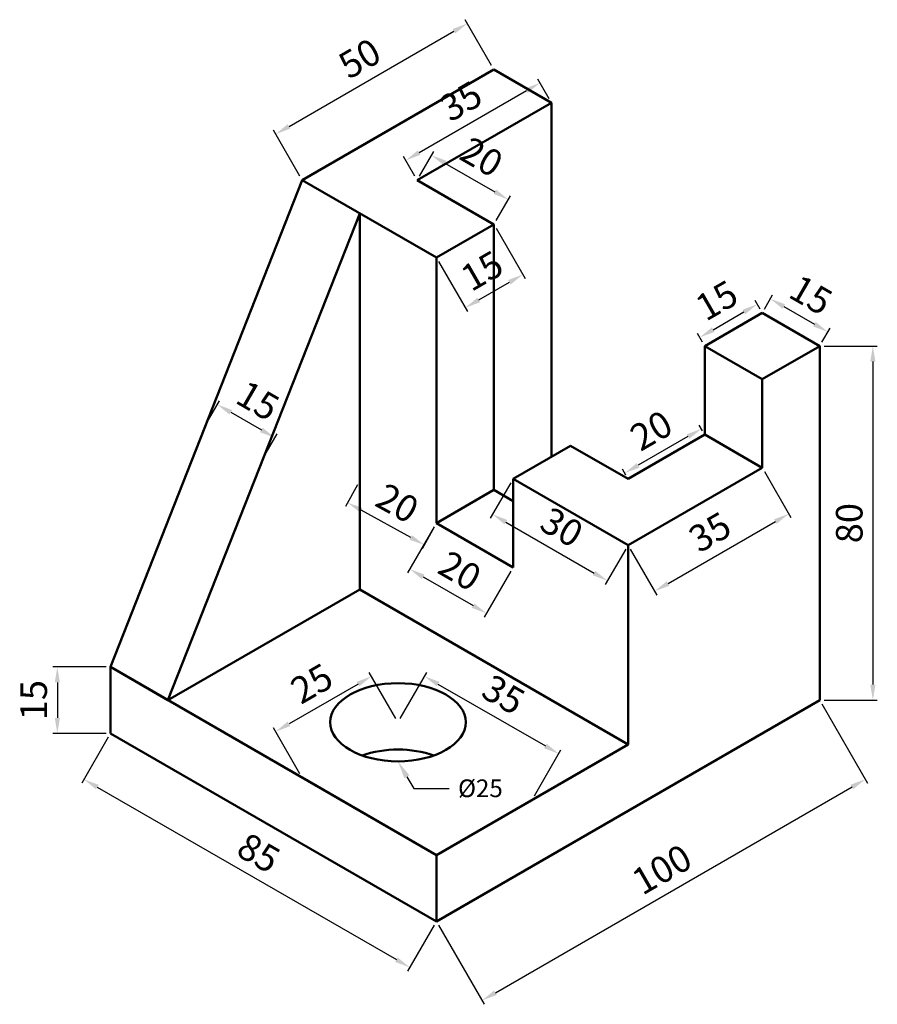
# Model space of a CAD drawing. Units: millimetres. Extents: x 2933 to 3127, y 771 to 994.
import ezdxf
from ezdxf import colors
from ezdxf.entities.mleader import LeaderData, LeaderLine
from ezdxf.math import Vec2, Vec3

# ---------------------------------------------------------------- set-up
doc = ezdxf.new("R2010")
doc.units = ezdxf.units.MM
for name, color, linetype, lineweight in [('M-DIMS', 3, 'Continuous', 25), ('M-OUTL', 7, 'Continuous', 50), ('M-TEXT', 7, 'Continuous', 25)]:
    doc.layers.add(name, color=color, linetype=linetype, lineweight=lineweight)
doc.styles.get("Standard").update_dxf_attribs({"font": 'arial.ttf'})
doc.dimstyles.new('AM_ISO$0', dxfattribs={"dimtxt": 6, "dimasz": 3.5, "dimexe": 1, "dimexo": 1, "dimgap": 1.5, "dimtad": 1, "dimdsep": 46, "dimtxsty": 'Standard', "dimcen": 0, "dimclrd": 256, "dimclre": 256, "dimclrt": 2, "dimadec": 0, "dimazin": 2, "dimtp": 0.1, "dimtm": 0.1, "dimtfac": 0.71, "dimtmove": 0, "dimatfit": 3, "dimfxl": 1, "dimlwd": -1, "dimlwe": -1, "dimarcsym": 1})

# ---------------------------------------------------------------- blocks, each defined once
blk = doc.blocks.new('*D3')
at = {"layer": 'Defpoints', "color": 0, "transparency": 16777216}
for p in [(3113.5, 839.77), (3123.82, 821.91), (3026.9, 789.77)]:
    blk.add_point(p, dxfattribs=at)
at = {"layer": 'M-DIMS', "color": 0, "linetype": 'ByBlock', "transparency": 16777216}
for p, q in [((3114, 838.9), (3124.32, 821.04)), ((3040.25, 773.66), (3120.79, 820.16)), ((3027.4, 788.9), (3037.71, 771.04))]:
    blk.add_line(p, q, dxfattribs=at)
at = {"layer": 'M-DIMS', "color": 0, "transparency": 16777216}
for points in [[(3120.49, 820.66), (3121.08, 819.65), (3123.82, 821.91)], [(3039.95, 774.16), (3040.54, 773.15), (3037.21, 771.91)]]:
    blk.add_solid(points, dxfattribs=at)
at = {"layer": 'M-DIMS', "color": 0, "transparency": 16777216, "insert": (3078.23, 800.86), "char_height": 6, "attachment_point": 5, "rotation": 30}
blk.add_mtext('100', dxfattribs=at)
blk = doc.blocks.new('*D4')
at = {"layer": 'Defpoints', "color": 0, "transparency": 16777216}
for p in [(3113.5, 919.77), (3113.5, 839.77), (3125.5, 839.77)]:
    blk.add_point(p, dxfattribs=at)
at = {"layer": 'M-DIMS', "color": 0, "linetype": 'ByBlock', "transparency": 16777216}
for p, q in [((3114.5, 919.77), (3126.5, 919.77)), ((3125.5, 916.27), (3125.5, 843.27)), ((3114.5, 839.77), (3126.5, 839.77))]:
    blk.add_line(p, q, dxfattribs=at)
at = {"layer": 'M-DIMS', "color": 0, "transparency": 16777216}
for points in [[(3124.92, 916.27), (3126.09, 916.27), (3125.5, 919.77)], [(3124.92, 843.27), (3126.09, 843.27), (3125.5, 839.77)]]:
    blk.add_solid(points, dxfattribs=at)
at = {"layer": 'M-DIMS', "color": 0, "transparency": 16777216, "insert": (3120.94, 879.77), "char_height": 6, "attachment_point": 5, "rotation": 90}
blk.add_mtext('80', dxfattribs=at)
blk = doc.blocks.new('*D5')
at = {"layer": 'Defpoints', "color": 0, "transparency": 16777216}
for p in [(2953.29, 832.27), (3026.9, 789.77), (3020.9, 779.38)]:
    blk.add_point(p, dxfattribs=at)
at = {"layer": 'M-DIMS', "color": 0, "linetype": 'ByBlock', "transparency": 16777216}
for p, q in [((2952.79, 831.4), (2946.79, 821.01)), ((2950.32, 820.13), (3017.87, 781.13)), ((3026.4, 788.9), (3020.4, 778.51))]:
    blk.add_line(p, q, dxfattribs=at)
at = {"layer": 'M-DIMS', "color": 0, "transparency": 16777216}
for points in [[(2950.61, 820.63), (2950.03, 819.62), (2947.29, 821.88)], [(3018.16, 781.63), (3017.58, 780.62), (3020.9, 779.38)]]:
    blk.add_solid(points, dxfattribs=at)
at = {"layer": 'M-DIMS', "color": 0, "transparency": 16777216, "insert": (2986.38, 804.58), "char_height": 6, "attachment_point": 5, "rotation": 330}
blk.add_mtext('85', dxfattribs=at)
blk = doc.blocks.new('*D6')
at = {"layer": 'Defpoints', "color": 0, "transparency": 16777216}
for p in [(2953.29, 847.27), (2941.29, 832.27), (2953.29, 832.27)]:
    blk.add_point(p, dxfattribs=at)
at = {"layer": 'M-DIMS', "color": 0, "linetype": 'ByBlock', "transparency": 16777216}
for p, q in [((2952.29, 847.27), (2940.29, 847.27)), ((2941.29, 843.77), (2941.29, 835.77)), ((2952.29, 832.27), (2940.29, 832.27))]:
    blk.add_line(p, q, dxfattribs=at)
at = {"layer": 'M-DIMS', "color": 0, "transparency": 16777216}
for points in [[(2940.71, 843.77), (2941.87, 843.77), (2941.29, 847.27)], [(2940.71, 835.77), (2941.87, 835.77), (2941.29, 832.27)]]:
    blk.add_solid(points, dxfattribs=at)
at = {"layer": 'M-DIMS', "color": 0, "transparency": 16777216, "insert": (2936.73, 839.77), "char_height": 6, "attachment_point": 5, "rotation": 90}
blk.add_mtext('15', dxfattribs=at)
blk = doc.blocks.new('*D7')
at = {"layer": 'Defpoints', "color": 0, "transparency": 16777216}
for p in [(3033.89, 992.66), (3039.89, 982.27), (2996.59, 957.27)]:
    blk.add_point(p, dxfattribs=at)
at = {"layer": 'M-DIMS', "color": 0, "linetype": 'ByBlock', "transparency": 16777216}
for p, q in [((3039.39, 983.14), (3033.39, 993.53)), ((2993.62, 969.41), (3030.86, 990.91)), ((2996.09, 958.14), (2990.09, 968.53))]:
    blk.add_line(p, q, dxfattribs=at)
at = {"layer": 'M-DIMS', "color": 0, "transparency": 16777216}
for points in [[(3030.57, 991.42), (3031.15, 990.41), (3033.89, 992.66)], [(2993.33, 969.92), (2993.91, 968.91), (2990.59, 967.66)]]:
    blk.add_solid(points, dxfattribs=at)
at = {"layer": 'M-DIMS', "color": 0, "transparency": 16777216, "insert": (3009.96, 984.11), "char_height": 6, "attachment_point": 5, "rotation": 30}
blk.add_mtext('50', dxfattribs=at)
blk = doc.blocks.new('*D8')
at = {"layer": 'Defpoints', "color": 0, "transparency": 16777216}
for p in [(3039.89, 947.27), (3026.9, 939.77), (3046.43, 935.94)]:
    blk.add_point(p, dxfattribs=at)
at = {"layer": 'M-DIMS', "color": 0, "linetype": 'ByBlock', "transparency": 16777216}
for p, q in [((3040.39, 946.4), (3046.93, 935.08)), ((3027.4, 938.9), (3033.94, 927.58)), ((3036.47, 930.19), (3043.4, 934.19))]:
    blk.add_line(p, q, dxfattribs=at)
at = {"layer": 'M-DIMS', "color": 0, "transparency": 16777216}
for points in [[(3043.11, 934.7), (3043.69, 933.69), (3046.43, 935.94)], [(3036.18, 930.7), (3036.76, 929.69), (3033.44, 928.44)]]:
    blk.add_solid(points, dxfattribs=at)
at = {"layer": 'M-DIMS', "color": 0, "transparency": 16777216, "insert": (3037.61, 936.12), "char_height": 6, "attachment_point": 5, "rotation": 30}
blk.add_mtext('15', dxfattribs=at)
blk = doc.blocks.new('*D9')
at = {"layer": 'Defpoints', "color": 0, "transparency": 16777216}
for p in [(3050.3, 979.25), (3052.88, 974.77), (3022.57, 957.27)]:
    blk.add_point(p, dxfattribs=at)
at = {"layer": 'M-DIMS', "color": 0, "linetype": 'ByBlock', "transparency": 16777216}
for p, q in [((3052.38, 975.64), (3049.8, 980.11)), ((3023.02, 963.5), (3047.27, 977.5)), ((3022.07, 958.14), (3019.49, 962.61))]:
    blk.add_line(p, q, dxfattribs=at)
at = {"layer": 'M-DIMS', "color": 0, "transparency": 16777216}
for points in [[(3046.98, 978), (3047.56, 976.99), (3050.3, 979.25)], [(3022.73, 964), (3023.31, 962.99), (3019.99, 961.75)]]:
    blk.add_solid(points, dxfattribs=at)
at = {"layer": 'M-DIMS', "color": 0, "transparency": 16777216, "insert": (3032.86, 974.45), "char_height": 6, "attachment_point": 5, "rotation": 30}
blk.add_mtext('35', dxfattribs=at)
blk = doc.blocks.new('*D10')
at = {"layer": 'Defpoints', "color": 0, "transparency": 16777216}
for p in [(3022.57, 957.27), (3043.14, 952.89), (3039.89, 947.27)]:
    blk.add_point(p, dxfattribs=at)
at = {"layer": 'M-DIMS', "color": 0, "linetype": 'ByBlock', "transparency": 16777216}
for p, q in [((3023.07, 958.14), (3026.32, 963.76)), ((3028.85, 961.14), (3040.11, 954.64)), ((3040.39, 948.14), (3043.64, 953.76))]:
    blk.add_line(p, q, dxfattribs=at)
at = {"layer": 'M-DIMS', "color": 0, "transparency": 16777216}
for points in [[(3029.14, 961.65), (3028.56, 960.64), (3025.82, 962.89)], [(3040.4, 955.15), (3039.82, 954.14), (3043.14, 952.89)]]:
    blk.add_solid(points, dxfattribs=at)
at = {"layer": 'M-DIMS', "color": 0, "transparency": 16777216, "insert": (3036.76, 961.85), "char_height": 6, "attachment_point": 5, "rotation": 330}
blk.add_mtext('20', dxfattribs=at)
blk = doc.blocks.new('*D11')
at = {"layer": 'Defpoints', "color": 0, "transparency": 16777216}
for p in [(3018.24, 834.77), (2990.59, 832.66), (2996.59, 822.27)]:
    blk.add_point(p, dxfattribs=at)
at = {"layer": 'M-DIMS', "color": 0, "linetype": 'ByBlock', "transparency": 16777216}
for p, q in [((3017.74, 835.64), (3011.74, 846.03)), ((3009.21, 843.41), (2993.62, 834.41)), ((2996.09, 823.14), (2990.09, 833.53))]:
    blk.add_line(p, q, dxfattribs=at)
at = {"layer": 'M-DIMS', "color": 0, "transparency": 16777216}
for points in [[(3008.92, 843.92), (3009.5, 842.91), (3012.24, 845.16)], [(2993.33, 834.92), (2993.91, 833.91), (2990.59, 832.66)]]:
    blk.add_solid(points, dxfattribs=at)
at = {"layer": 'M-DIMS', "color": 0, "transparency": 16777216, "insert": (2999.13, 842.86), "char_height": 6, "attachment_point": 5, "rotation": 30}
blk.add_mtext('25', dxfattribs=at)
blk = doc.blocks.new('*D12')
at = {"layer": 'Defpoints', "color": 0, "transparency": 16777216}
for p in [(3018.24, 834.77), (3054.55, 827.66), (3048.55, 817.27)]:
    blk.add_point(p, dxfattribs=at)
at = {"layer": 'M-DIMS', "color": 0, "linetype": 'ByBlock', "transparency": 16777216}
for p, q in [((3018.74, 835.64), (3024.74, 846.03)), ((3027.27, 843.41), (3051.52, 829.41)), ((3049.05, 818.14), (3055.05, 828.53))]:
    blk.add_line(p, q, dxfattribs=at)
at = {"layer": 'M-DIMS', "color": 0, "transparency": 16777216}
for points in [[(3027.56, 843.92), (3026.98, 842.91), (3024.24, 845.16)], [(3051.81, 829.92), (3051.23, 828.91), (3054.55, 827.66)]]:
    blk.add_solid(points, dxfattribs=at)
at = {"layer": 'M-DIMS', "color": 0, "transparency": 16777216, "insert": (3041.68, 840.37), "char_height": 6, "attachment_point": 5, "rotation": 330}
blk.add_mtext('35', dxfattribs=at)
blk = doc.blocks.new('*D13')
at = {"layer": 'Defpoints', "color": 0, "transparency": 16777216}
for p in [(3044.22, 889.77), (3070.2, 874.77), (3065.57, 866.74)]:
    blk.add_point(p, dxfattribs=at)
at = {"layer": 'M-DIMS', "color": 0, "linetype": 'ByBlock', "transparency": 16777216}
for p, q in [((3043.72, 888.9), (3039.09, 880.87)), ((3042.62, 879.99), (3062.54, 868.49)), ((3069.7, 873.9), (3065.07, 865.87))]:
    blk.add_line(p, q, dxfattribs=at)
at = {"layer": 'M-DIMS', "color": 0, "transparency": 16777216}
for points in [[(3042.91, 880.49), (3042.32, 879.48), (3039.59, 881.74)], [(3062.83, 868.99), (3062.24, 867.98), (3065.57, 866.74)]]:
    blk.add_solid(points, dxfattribs=at)
at = {"layer": 'M-DIMS', "color": 0, "transparency": 16777216, "insert": (3054.86, 878.19), "char_height": 6, "attachment_point": 5, "rotation": 330}
blk.add_mtext('30', dxfattribs=at)
blk = doc.blocks.new('*D14')
at = {"layer": 'Defpoints', "color": 0, "transparency": 16777216}
for p in [(3026.9, 879.77), (3044.22, 869.77), (3038.22, 859.38)]:
    blk.add_point(p, dxfattribs=at)
at = {"layer": 'M-DIMS', "color": 0, "linetype": 'ByBlock', "transparency": 16777216}
for p, q in [((3026.4, 878.9), (3020.4, 868.51)), ((3043.72, 868.9), (3037.72, 858.51)), ((3023.93, 867.63), (3035.19, 861.13))]:
    blk.add_line(p, q, dxfattribs=at)
at = {"layer": 'M-DIMS', "color": 0, "transparency": 16777216}
for points in [[(3024.22, 868.13), (3023.64, 867.12), (3020.9, 869.38)], [(3035.48, 861.63), (3034.9, 860.62), (3038.22, 859.38)]]:
    blk.add_solid(points, dxfattribs=at)
at = {"layer": 'M-DIMS', "color": 0, "transparency": 16777216, "insert": (3031.84, 868.33), "char_height": 6, "attachment_point": 5, "rotation": 330}
blk.add_mtext('20', dxfattribs=at)
blk = doc.blocks.new('*D15')
at = {"layer": 'Defpoints', "color": 0, "transparency": 16777216}
for p in [(3009.58, 889.31), (3006.87, 884.38), (3026.9, 879.77)]:
    blk.add_point(p, dxfattribs=at)
at = {"layer": 'M-DIMS', "color": 0, "linetype": 'ByBlock', "transparency": 16777216}
for p, q in [((3009.1, 888.43), (3006.39, 883.51)), ((3021.12, 876.53), (3009.94, 882.7)), ((3026.42, 878.89), (3023.71, 873.97))]:
    blk.add_line(p, q, dxfattribs=at)
at = {"layer": 'M-DIMS', "color": 0, "transparency": 16777216}
for points in [[(3010.22, 883.21), (3009.65, 882.18), (3006.87, 884.38)], [(3021.41, 877.04), (3020.84, 876.02), (3024.19, 874.84)]]:
    blk.add_solid(points, dxfattribs=at)
at = {"layer": 'M-DIMS', "color": 0, "transparency": 16777216, "insert": (3017.73, 883.61), "char_height": 6, "attachment_point": 5, "rotation": 331.1574}
blk.add_mtext('20', dxfattribs=at)
blk = doc.blocks.new('*D16')
at = {"layer": 'Defpoints', "color": 0, "transparency": 16777216}
for p in [(3100.51, 892.27), (3106.51, 881.88), (3070.2, 874.77)]:
    blk.add_point(p, dxfattribs=at)
at = {"layer": 'M-DIMS', "color": 0, "linetype": 'ByBlock', "transparency": 16777216}
for p, q in [((3101.01, 891.4), (3107.01, 881.01)), ((3079.23, 866.13), (3103.48, 880.13)), ((3070.7, 873.9), (3076.7, 863.51))]:
    blk.add_line(p, q, dxfattribs=at)
at = {"layer": 'M-DIMS', "color": 0, "transparency": 16777216}
for points in [[(3103.19, 880.63), (3103.77, 879.62), (3106.51, 881.88)], [(3078.94, 866.63), (3079.53, 865.62), (3076.2, 864.38)]]:
    blk.add_solid(points, dxfattribs=at)
at = {"layer": 'M-DIMS', "color": 0, "transparency": 16777216, "insert": (3089.08, 877.08), "char_height": 6, "attachment_point": 5, "rotation": 30}
blk.add_mtext('35', dxfattribs=at)
blk = doc.blocks.new('*D17')
at = {"layer": 'Defpoints', "color": 0, "transparency": 16777216}
for p in [(3099.38, 929.23), (3100.51, 927.27), (3087.52, 919.77)]:
    blk.add_point(p, dxfattribs=at)
at = {"layer": 'M-DIMS', "color": 0, "linetype": 'ByBlock', "transparency": 16777216}
for p, q in [((3100.01, 928.14), (3098.88, 930.1)), ((3089.42, 923.48), (3096.35, 927.48)), ((3087.02, 920.64), (3085.89, 922.6))]:
    blk.add_line(p, q, dxfattribs=at)
at = {"layer": 'M-DIMS', "color": 0, "transparency": 16777216}
for points in [[(3096.06, 927.98), (3096.64, 926.97), (3099.38, 929.23)], [(3089.13, 923.98), (3089.72, 922.97), (3086.39, 921.73)]]:
    blk.add_solid(points, dxfattribs=at)
at = {"layer": 'M-DIMS', "color": 0, "transparency": 16777216, "insert": (3090.61, 929.43), "char_height": 6, "attachment_point": 5, "rotation": 30}
blk.add_mtext('15', dxfattribs=at)
blk = doc.blocks.new('*D18')
at = {"layer": 'Defpoints', "color": 0, "transparency": 16777216}
for p in [(3100.51, 927.27), (3115.35, 922.96), (3113.5, 919.77)]:
    blk.add_point(p, dxfattribs=at)
at = {"layer": 'M-DIMS', "color": 0, "linetype": 'ByBlock', "transparency": 16777216}
for p, q in [((3101.01, 928.14), (3102.86, 931.33)), ((3105.39, 928.71), (3112.32, 924.71)), ((3114, 920.64), (3115.85, 923.83))]:
    blk.add_line(p, q, dxfattribs=at)
at = {"layer": 'M-DIMS', "color": 0, "transparency": 16777216}
for points in [[(3105.68, 929.22), (3105.1, 928.21), (3102.36, 930.46)], [(3112.61, 925.22), (3112.03, 924.21), (3115.35, 922.96)]]:
    blk.add_solid(points, dxfattribs=at)
at = {"layer": 'M-DIMS', "color": 0, "transparency": 16777216, "insert": (3111.13, 930.66), "char_height": 6, "attachment_point": 5, "rotation": 330}
blk.add_mtext('15', dxfattribs=at)
blk = doc.blocks.new('*D19')
at = {"layer": 'Defpoints', "color": 0, "transparency": 16777216}
for p in [(2974.94, 902.27), (2990.41, 899.07), (2987.93, 894.77)]:
    blk.add_point(p, dxfattribs=at)
at = {"layer": 'M-DIMS', "color": 0, "linetype": 'ByBlock', "transparency": 16777216}
for p, q in [((2975.44, 903.14), (2977.92, 907.44)), ((2980.45, 904.82), (2987.38, 900.82)), ((2988.43, 895.64), (2990.91, 899.94))]:
    blk.add_line(p, q, dxfattribs=at)
at = {"layer": 'M-DIMS', "color": 0, "transparency": 16777216}
for points in [[(2980.75, 905.33), (2980.16, 904.32), (2977.42, 906.57)], [(2987.67, 901.33), (2987.09, 900.32), (2990.41, 899.07)]]:
    blk.add_solid(points, dxfattribs=at)
at = {"layer": 'M-DIMS', "color": 0, "transparency": 16777216, "insert": (2986.2, 906.77), "char_height": 6, "attachment_point": 5, "rotation": 330}
blk.add_mtext('15', dxfattribs=at)
blk = doc.blocks.new('*D20')
at = {"layer": 'Defpoints', "color": 0, "transparency": 16777216}
for p in [(3087.52, 899.77), (3069.45, 891.08), (3070.2, 889.77)]:
    blk.add_point(p, dxfattribs=at)
at = {"layer": 'M-DIMS', "color": 0, "linetype": 'ByBlock', "transparency": 16777216}
for p, q in [((3087.02, 900.64), (3086.27, 901.94)), ((3083.74, 899.33), (3072.48, 892.83)), ((3069.7, 890.64), (3068.95, 891.94))]:
    blk.add_line(p, q, dxfattribs=at)
at = {"layer": 'M-DIMS', "color": 0, "transparency": 16777216}
for points in [[(3083.45, 899.83), (3084.03, 898.82), (3086.77, 901.08)], [(3072.19, 893.33), (3072.77, 892.32), (3069.45, 891.08)]]:
    blk.add_solid(points, dxfattribs=at)
at = {"layer": 'M-DIMS', "color": 0, "transparency": 16777216, "insert": (3075.83, 900.03), "char_height": 6, "attachment_point": 5, "rotation": 30}
blk.add_mtext('20', dxfattribs=at)

msp = doc.modelspace()

# ---------------------------------------------------------------- linework, layer by layer
at = {"layer": 'M-OUTL'}
for p, q in [((3039.892, 982.269), (2996.591, 957.269)), ((3052.883, 974.769), (3039.892, 982.269)), ((3022.572, 957.269), (3052.883, 974.769)), ((3052.883, 974.769), (3052.883, 894.769)), ((2953.29, 847.269), (2996.591, 957.269)), ((2996.591, 957.269), (3026.902, 939.769)), ((3039.892, 947.269), (3022.572, 957.269)), ((2966.28, 839.769), (3009.582, 949.769)), ((3009.582, 864.769), (3009.582, 949.769)), ((3026.902, 939.769), (3039.892, 947.269)), ((3039.892, 947.269), (3039.892, 887.269)), ((3026.902, 879.769), (3026.902, 939.769)), ((3087.524, 919.769), (3100.514, 927.269)), ((3100.514, 927.269), (3113.505, 919.769)), ((3100.514, 912.269), (3087.524, 919.769)), ((3087.524, 899.769), (3087.524, 919.769)), ((3113.505, 919.769), (3100.514, 912.269)), ((3113.505, 839.769), (3113.505, 919.769)), ((3100.514, 912.269), (3100.514, 892.269)), ((3087.524, 899.769), (3070.203, 889.769)), ((3100.514, 892.269), (3087.524, 899.769)), ((3057.213, 897.269), (3044.223, 889.769)), ((3070.203, 889.769), (3057.213, 897.269)), ((3100.514, 892.269), (3070.203, 874.769)), ((3044.223, 889.769), (3070.203, 874.769)), ((3044.223, 889.769), (3044.223, 869.769)), ((3026.902, 879.769), (3039.892, 887.269)), ((3039.892, 887.269), (3044.223, 884.769)), ((3044.223, 869.769), (3026.902, 879.769)), ((3070.203, 874.769), (3070.203, 829.769)), ((2966.28, 839.769), (3009.582, 864.769)), ((3070.203, 829.769), (3009.582, 864.769)), ((2953.29, 832.269), (2953.29, 847.269)), ((2953.29, 847.269), (3026.902, 804.769)), ((2953.29, 847.269), (2966.28, 839.769)), ((3026.902, 789.769), (3113.505, 839.769)), ((3026.902, 789.769), (2953.29, 832.269)), ((3026.902, 804.769), (3070.203, 829.769)), ((3026.902, 804.769), (2996.591, 822.269)), ((3026.902, 789.769), (3026.902, 804.769))]:
    msp.add_line(p, q, dxfattribs=at)
msp.add_ellipse((3018.242, 834.769), major_axis=(-15.309, 0), ratio=0.5773503, dxfattribs=at)
msp.add_ellipse((3018.242, 819.769), major_axis=(-15.309, 0), ratio=0.5773503, start_param=4.1547902, end_param=5.2699878, dxfattribs=at)

# ---------------------------------------------------------------- dimensions: what is measured, and where the dimension line sits
at = {"layer": 'M-DIMS'}
for p1, p2, distance, override, picture, middle in [((2996.591, 957.269), (3039.892, 982.269), 12, {"dimclrd": 0, "dimclre": 0, "dimclrt": 0}, '*D7', (3009.96, 984.113)), ((3022.572, 957.269), (3052.883, 974.769), 5.169, {"dimclrd": 0, "dimclre": 0, "dimclrt": 0}, '*D9', (3032.86, 974.449)), ((3022.572, 957.269), (3039.892, 947.269), 6.495, {"dimclrd": 0, "dimclre": 0, "dimclrt": 0}, '*D10', (3036.761, 961.846)), ((3087.524, 919.769), (3100.514, 927.269), 2.263, {"dimclrd": 0, "dimclre": 0, "dimclrt": 0}, '*D17', (3090.606, 929.431)), ((3100.514, 927.269), (3113.505, 919.769), 3.686, {"dimclrd": 0, "dimclre": 0, "dimclrt": 0}, '*D18', (3111.134, 930.664)), ((3113.505, 919.769), (3113.505, 839.769), 12, {"dimclrd": 0, "dimclre": 0, "dimclrt": 0}, '*D4', (3120.941, 879.769)), ((2974.941, 902.269), (2987.931, 894.769), 4.966, {"dimpost": '', "dimclrd": 0, "dimclre": 0, "dimclrt": 0}, '*D19', (2986.201, 906.772)), ((3087.524, 899.769), (3070.203, 889.769), -1.51, {"dimpost": '', "dimclrd": 0, "dimclre": 0, "dimclrt": 0}, '*D20', (3075.827, 900.029)), ((3070.203, 874.769), (3100.514, 892.269), -12, {"dimpost": '', "dimclrd": 0, "dimclre": 0, "dimclrt": 0}, '*D16', (3089.076, 877.081)), ((3026.902, 879.769), (3044.223, 869.769), -12, {"dimclrd": 0, "dimclre": 0, "dimclrt": 0}, '*D14', (3031.844, 868.329)), ((3018.242, 834.769), (2996.591, 822.269), -12, {"dimclrd": 0, "dimclre": 0, "dimclrt": 0}, '*D11', (2999.135, 842.863)), ((2953.29, 847.269), (2953.29, 832.269), -12, {"dimclrd": 0, "dimclre": 0, "dimclrt": 0}, '*D6', (2936.726, 839.769)), ((3018.242, 834.769), (3048.553, 817.269), 12, {"dimclrd": 0, "dimclre": 0, "dimclrt": 0}, '*D12', (3041.68, 840.365)), ((3026.902, 789.769), (3113.505, 839.769), -20.625, {"dimpost": '', "dimclrd": 0, "dimclre": 0, "dimclrt": 0}, '*D3', (3078.234, 800.859)), ((2953.29, 832.269), (3026.902, 789.769), -12, {"dimclrd": 0, "dimclre": 0, "dimclrt": 0}, '*D5', (2986.378, 804.579))]:
    dim = msp.add_aligned_dim(p1=p1, p2=p2, distance=distance, dimstyle='AM_ISO$0', override=override, dxfattribs=at)
    dim.commit()
    dim.dimension.update_dxf_attribs({"geometry": picture, "text_midpoint": middle})
for base, p1, p2, angle, picture, middle in [((3046.432, 935.942), (3026.902, 939.769), (3039.892, 947.269), 30, '*D8', (3039.892, 932.166)), ((3065.566, 866.737), (3044.223, 889.769), (3070.203, 874.769), 330, '*D13', (3052.576, 874.237))]:
    dim = msp.add_linear_dim(base=base, p1=p1, p2=p2, angle=angle, dimstyle='AM_ISO$0', override={"dimclrd": 0, "dimclre": 0, "dimclrt": 0}, dxfattribs=at)
    dim.commit()
    dim.dimension.update_dxf_attribs({"geometry": picture, "text_midpoint": middle, "dimtype": 161})
dim = msp.add_aligned_dim(p1=(3026.902, 879.769), p2=(3009.582, 889.308), distance=5.622, text='20', dimstyle='AM_ISO$0', override={"dimpost": '', "dimclrd": 0, "dimclre": 0, "dimclrt": 0}, dxfattribs=at)
dim.commit()
dim.dimension.update_dxf_attribs({"geometry": '*D15', "text_midpoint": (3017.731, 883.611)})

# ---------------------------------------------------------------- leaders
at = {"layer": 'M-TEXT'}
ml = msp.add_multileader_mtext('Standard', dxfattribs=at)
ml.set_content('{\\C2;%%C25}', color=256)
ml.set_leader_properties()
ml.build(insert=Vec2(0, 0))
ctx = ml.context
ctx.base_point, ctx.plane_origin = Vec3(3029.799, 819.769), Vec3(3018.242, 825.93)
notes = []
notes.append((ctx, [(0, (1, 1, 0), (3021.799, 819.769), (1, 0), 8, [(0, [(3018.242, 825.93)], 0, [])])]))
ctx.mtext.insert, ctx.mtext.flow_direction = Vec3(3031.799, 821.85), 5
for ctx, leaders in notes:
    for number, flags, end, landing, length, lines in leaders:
        leader = LeaderData()
        leader.index, (leader.has_last_leader_line, leader.has_dogleg_vector, leader.attachment_direction) = number, flags
        leader.last_leader_point, leader.dogleg_vector, leader.dogleg_length = Vec3(end), Vec3(landing), length
        for number, points, colour, breaks in lines:
            line = LeaderLine()
            line.index, line.vertices, line.color, line.breaks = number, Vec3.list(points), colors.encode_raw_color(colour), breaks
            leader.lines.append(line)
        ctx.leaders.append(leader)

doc.saveas('drawing.dxf')
